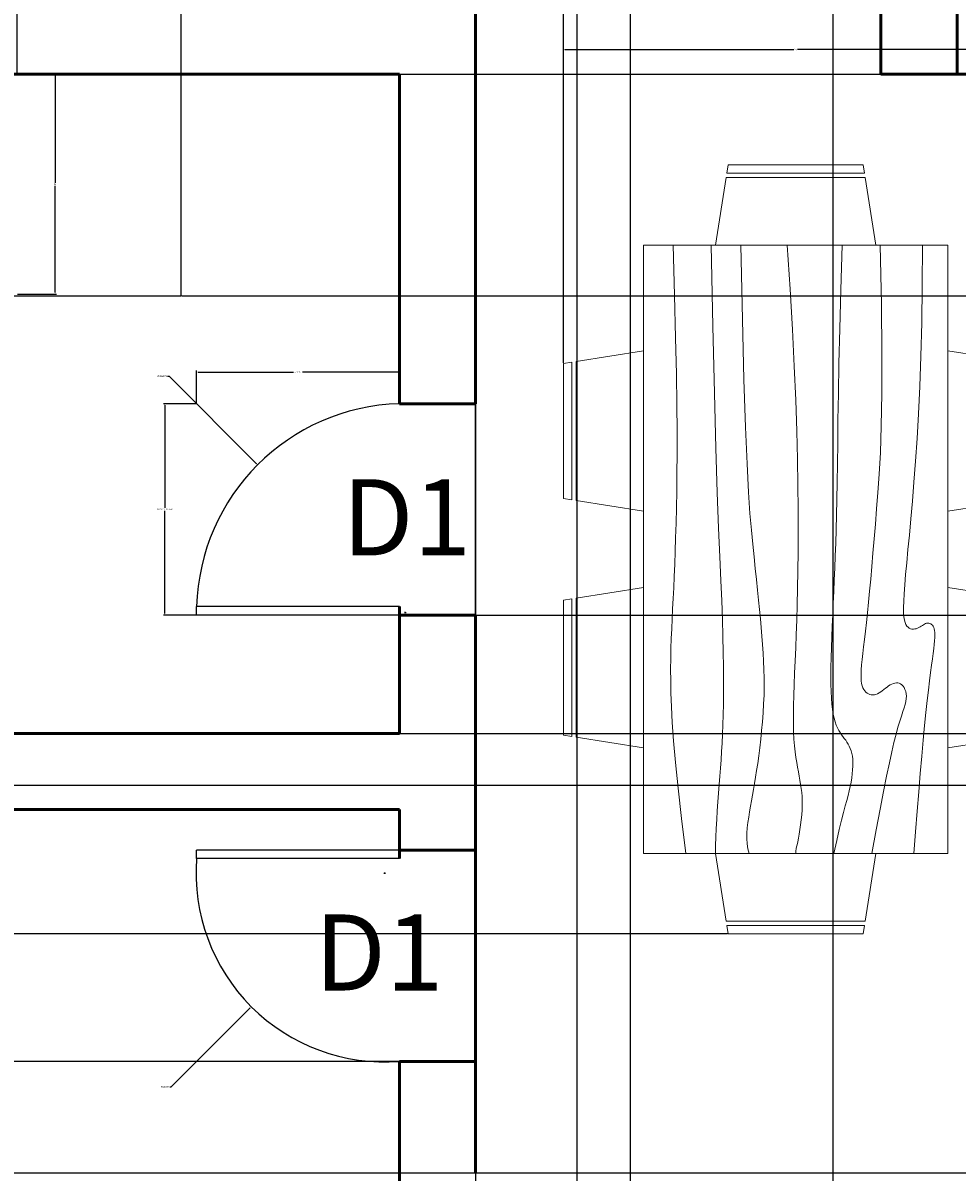
# Model space of a CAD drawing. Units: inches. Extents: x -3 to 419, y -430 to 101.
# Tile 3 of 5: x 118 to 229, y -259 to -123. Entities that reach past the tile are written whole.
import ezdxf

# ---------------------------------------------------------------- set-up
doc = ezdxf.new("R2010")
doc.units = ezdxf.units.IN
doc.header["$MEASUREMENT"] = 0
for name, color, linetype, lineweight in [('A-ANNO-DIMS', 2, 'Continuous', 18), ('A-ANNO-TEXT', 7, 'Continuous', 18), ('A-DOOR', 3, 'Continuous', 25), ('A-FLOR-CASE', 9, 'Continuous', 25), ('A-FURN', 8, 'Continuous', 18), ('A-WALL', 7, 'Continuous', 50)]:
    doc.layers.add(name, color=color, linetype=linetype, lineweight=lineweight)
doc.styles.get("Standard").update_dxf_attribs({"font": 'arial.ttf'})
doc.dimstyles.get("Standard").update_dxf_attribs({"dimtxt": 0.18, "dimasz": 0.18, "dimexe": 0.18, "dimexo": 0.0625, "dimgap": 0.09, "dimtad": 0, "dimtih": 1, "dimtoh": 1, "dimdec": 4, "dimzin": 0, "dimdsep": 46, "dimtxsty": 'Standard', "dimcen": 0.09, "dimadec": 0, "dimazin": 0, "dimtfac": 1, "dimtdec": 4, "dimtofl": 0, "dimtmove": 0, "dimatfit": 3, "dimfxl": 1, "dimtolj": 1, "dimtzin": 0, "dimarcsym": 0})

# ---------------------------------------------------------------- blocks, each defined once
blk = doc.blocks.new('Dining Set - 36 x 72 in.')
for p, q in [((-22, 27.5), (-22.1562, 26.50042)), ((-22, 27.5), (-6, 27.5)), ((-5.8437, 26.49966), (-6, 27.5)), ((6, 27.5), (5.8438, 26.50042)), ((6, 27.5), (22, 27.5)), ((22.1563, 26.49966), (22, 27.5)), ((-22.2343, 26.00059), (-23.4847, 17.99762)), ((-22.2304, 26), (-5.7608, 26)), ((-5.8416, 26.5), (-22.1534, 26.5)), ((-4.5152, 17.99762), (-5.7655, 25.99926)), ((5.7657, 26.00059), (4.5153, 17.99762)), ((5.7696, 26), (22.2392, 26)), ((22.1584, 26.5), (5.8466, 26.5)), ((23.4848, 17.99762), (22.2345, 25.99926)), ((36, 18), (-36, 18)), ((-36, 18), (-36, -18)), ((36, -18), (36, 18)), ((-44.0006, 8.23428), (-35.9976, 9.48474)), ((-44, 8.23041), (-44, -8.23915)), ((44.0006, 8.23428), (35.9976, 9.48474)), ((44, 8.23041), (44, -8.23915)), ((-45.5, 8), (-44.5004, 8.15617)), ((-45.5, 8), (-45.5, -8)), ((-44.5, -8.15843), (-44.5, 8.15338)), ((44.5, -8.15843), (44.5, 8.15338)), ((45.5, 8), (44.5005, 8.15617)), ((45.5, 8), (45.5, -8)), ((-44.4997, -8.15631), (-45.5, -8)), ((44.4997, -8.15631), (45.5, -8)), ((-35.9976, -9.48476), (-43.9993, -8.2345)), ((35.9976, -9.48476), (43.9993, -8.2345)), ((-36, -18), (36, -18)), ((-22.2343, -26.0006), (-23.4847, -17.99762)), ((-4.5152, -17.99762), (-5.7655, -25.99928)), ((5.7657, -26.0006), (4.5153, -17.99762)), ((23.4848, -17.99762), (22.2345, -25.99928)), ((-22.2304, -26), (-5.7608, -26)), ((-22, -27.5), (-22.1562, -26.50044)), ((-5.8416, -26.5), (-22.1534, -26.5)), ((-5.8437, -26.49967), (-6, -27.5)), ((5.7696, -26), (22.2392, -26)), ((6, -27.5), (5.8438, -26.50044)), ((22.1584, -26.5), (5.8466, -26.5)), ((22.1563, -26.49967), (22, -27.5)), ((-22, -27.5), (-6, -27.5)), ((6, -27.5), (22, -27.5))]:
    blk.add_line(p, q)
for points in [[(-36, 15), (-31.1772, 14.97754), (-26.8079, 14.91406), (-22.8538, 14.81543), (-19.276, 14.6875), (-16.0362, 14.53613), (-13.0957, 14.36718), (-10.4159, 14.18652), (-7.9583, 14), (-5.6904, 13.81315), (-3.6035, 13.63021), (-1.6954, 13.45508), (0.0365, 13.29166), (1.5945, 13.14388), (2.9811, 13.01562), (4.1988, 12.9108), (5.25, 12.83333), (6.1393, 12.78613), (6.8802, 12.76823), (7.4883, 12.77767), (7.9792, 12.8125), (8.3685, 12.87077), (8.6719, 12.95052), (8.9049, 13.0498), (9.0833, 13.16666), (9.2205, 13.29899), (9.3216, 13.44401), (9.3895, 13.59879), (9.4271, 13.76041), (9.4373, 13.92594), (9.4232, 14.09245), (9.3875, 14.257), (9.3333, 14.41666), (9.2638, 14.56917), (9.1836, 14.71484), (9.0975, 14.85465), (9.0104, 14.98958), (8.9272, 15.1206), (8.8529, 15.2487), (8.7922, 15.37483), (8.75, 15.5), (8.7305, 15.62467), (8.7344, 15.74739), (8.7617, 15.86621), (8.8125, 15.97916), (8.8867, 16.08431), (8.9844, 16.17968), (9.1055, 16.26334), (9.25, 16.33333), (9.4189, 16.38802), (9.6172, 16.42708), (9.8506, 16.45052), (10.125, 16.45833), (10.4463, 16.45052), (10.8203, 16.42708), (11.2529, 16.38802), (11.75, 16.33333), (12.3184, 16.26318), (12.9694, 16.17838), (13.7151, 16.07991), (14.5677, 15.96875), (15.5395, 15.84586), (16.6426, 15.71224), (17.8893, 15.56884), (19.2917, 15.41666), (20.859, 15.25667), (22.5879, 15.08984), (24.4721, 14.91715), (26.5052, 14.73958), (28.6809, 14.5581), (30.9929, 14.3737), (33.4347, 14.18733), (36, 14)], [(-36, 10), (-28.9766, 10.14274), (-23.1725, 10.20442), (-18.4241, 10.19775), (-14.5677, 10.13541), (-11.4399, 10.03011), (-8.877, 9.89453), (-6.7154, 9.74137), (-4.7917, 9.58333), (-2.9698, 9.43082), (-1.2246, 9.28515), (0.4415, 9.14534), (2.026, 9.01041), (3.5266, 8.87939), (4.9408, 8.7513), (6.266, 8.62516), (7.5, 8.5), (8.6411, 8.37549), (9.6914, 8.2539), (10.6538, 8.13818), (11.5312, 8.03125), (12.3267, 7.93603), (13.043, 7.85547), (13.6831, 7.79248), (14.25, 7.75), (14.7471, 7.7303), (15.1797, 7.73307), (15.5537, 7.75732), (15.875, 7.80208), (16.1494, 7.86637), (16.3828, 7.94922), (16.5811, 8.04964), (16.75, 8.16666), (16.8944, 8.29915), (17.0143, 8.44531), (17.1089, 8.60319), (17.1771, 8.77083), (17.218, 8.94629), (17.2305, 9.1276), (17.2137, 9.31282), (17.1667, 9.5), (17.0895, 9.6875), (16.987, 9.875), (16.8649, 10.0625), (16.7292, 10.25), (16.5856, 10.4375), (16.4401, 10.625), (16.2985, 10.8125), (16.1667, 11), (16.05, 11.18733), (15.9518, 11.3737), (15.8752, 11.5581), (15.8229, 11.73958), (15.798, 11.91715), (15.8034, 12.08984), (15.842, 12.25667), (15.9167, 12.41666), (16.0295, 12.56836), (16.1784, 12.70833), (16.3605, 12.83268), (16.5729, 12.9375), (16.8127, 13.01888), (17.0768, 13.07291), (17.3625, 13.0957), (17.6667, 13.08333), (17.9894, 13.03312), (18.3418, 12.94726), (18.7382, 12.82918), (19.1927, 12.68229), (19.7195, 12.51001), (20.3327, 12.31575), (21.0465, 12.10294), (21.875, 11.875), (22.8357, 11.63354), (23.959, 11.37304), (25.2786, 11.08618), (26.8282, 10.76562), (28.6414, 10.40405), (30.752, 9.99414), (33.1936, 9.52856), (36, 9)], [(-36, 5.5), (-30.7157, 5.3348), (-26.069, 5.20963), (-21.9946, 5.11767), (-18.4271, 5.05208), (-15.3009, 5.00602), (-12.5508, 4.97265), (-10.1112, 4.94515), (-7.9167, 4.91666), (-5.909, 4.88167), (-4.0586, 4.83984), (-2.3429, 4.79215), (-0.7396, 4.73958), (0.7739, 4.6831), (2.22, 4.6237), (3.6213, 4.56233), (5, 4.5), (6.373, 4.43782), (7.7344, 4.3776), (9.0723, 4.32129), (10.375, 4.27083), (11.6309, 4.22819), (12.8281, 4.19531), (13.9551, 4.17415), (15, 4.16666), (15.954, 4.17448), (16.819, 4.19791), (17.6001, 4.23698), (18.3021, 4.29166), (18.9299, 4.36198), (19.4883, 4.44791), (19.9823, 4.54948), (20.4167, 4.66666), (20.7969, 4.79899), (21.1302, 4.94401), (21.4245, 5.09879), (21.6875, 5.26041), (21.9271, 5.42594), (22.1511, 5.59245), (22.3672, 5.757), (22.5834, 5.91666), (22.8065, 6.06868), (23.0404, 6.21093), (23.2879, 6.34147), (23.5521, 6.45833), (23.8358, 6.55957), (24.142, 6.64323), (24.4735, 6.70735), (24.8334, 6.75), (25.2235, 6.76969), (25.642, 6.76692), (26.0858, 6.74267), (26.5521, 6.69791), (27.0379, 6.63362), (27.5404, 6.55078), (28.0565, 6.45036), (28.5834, 6.33333), (29.1242, 6.19987), (29.7071, 6.04687), (30.3661, 5.87044), (31.1354, 5.66666), (32.0493, 5.43164), (33.142, 5.16146), (34.4475, 4.85221), (36, 4.5)], [(-36, -1), (-30.7915, -0.6591), (-26.0195, -0.38216), (-21.6519, -0.16284), (-17.6563, 0.00521), (-14.0005, 0.12833), (-10.6523, 0.21289), (-7.5796, 0.26522), (-4.75, 0.29166), (-2.134, 0.29793), (0.2878, 0.28711), (2.5317, 0.26163), (4.6146, 0.22396), (6.5529, 0.17651), (8.3633, 0.12174), (10.0623, 0.06209), (11.6667, 0), (13.1899, -0.06201), (14.6341, -0.1211), (15.9982, -0.17432), (17.2813, -0.21875), (18.4823, -0.25147), (19.6003, -0.26953), (20.6343, -0.27002), (21.5834, -0.25), (22.4481, -0.20768), (23.2357, -0.14584), (23.9549, -0.06836), (24.6146, 0.02083), (25.2235, 0.11784), (25.7904, 0.21875), (26.3241, 0.31966), (26.8334, 0.41666), (27.3265, 0.50618), (27.8099, 0.58593), (28.2894, 0.65397), (28.7709, 0.70833), (29.2601, 0.74707), (29.763, 0.76823), (30.2855, 0.76985), (30.8334, 0.75), (31.4088, 0.70784), (31.9994, 0.64713), (32.589, 0.57275), (33.1615, 0.48958), (33.7008, 0.4025), (34.1908, 0.3164), (34.6153, 0.23616), (34.9584, 0.16666), (35.2099, 0.11165), (35.3848, 0.07031), (35.504, 0.04069), (35.5886, 0.02083), (35.6594, 0.00879), (35.7377, 0.0026), (35.8442, 0.00032), (36, 0)], [(-36, -6.5), (-27.1843, -6.31267), (-20.084, -6.1263), (-14.469, -5.9419), (-10.1094, -5.76042), (-6.7752, -5.58285), (-4.2363, -5.41016), (-2.2629, -5.24333), (-0.625, -5.08334), (0.8708, -4.93099), (2.2715, -4.78646), (3.5872, -4.64974), (4.8281, -4.52084), (6.0046, -4.39974), (7.127, -4.28646), (8.2053, -4.18099), (9.25, -4.08334), (10.2705, -3.99382), (11.2734, -3.91407), (12.2647, -3.84603), (13.25, -3.79167), (14.2354, -3.75293), (15.2266, -3.73177), (16.2295, -3.73015), (17.25, -3.75), (18.2912, -3.79248), (19.3451, -3.85547), (20.4009, -3.93604), (21.4479, -4.03125), (22.4754, -4.13819), (23.4727, -4.25391), (24.4289, -4.37549), (25.3334, -4.5), (26.1785, -4.62492), (26.9694, -4.74935), (27.7145, -4.87281), (28.4219, -4.99479), (29.1, -5.11483), (29.7572, -5.23242), (30.4016, -5.34709), (31.0417, -5.45834), (31.6837, -5.56437), (32.3262, -5.65821), (32.9658, -5.73153), (33.599, -5.77604), (34.2224, -5.78345), (34.8327, -5.74545), (35.4264, -5.65373), (36, -5.5)], [(-36, -10), (-26.4022, -9.81299), (-18.4675, -9.62891), (-11.9839, -9.45069), (-6.7396, -9.28125), (-2.5226, -9.12354), (0.8789, -8.98047), (3.6769, -8.85498), (6.0833, -8.75), (8.2767, -8.66765), (10.3021, -8.60677), (12.1712, -8.56543), (13.8958, -8.54167), (15.4876, -8.53353), (16.9583, -8.53907), (18.3197, -8.55632), (19.5834, -8.58334), (20.7616, -8.61841), (21.8685, -8.66081), (22.9188, -8.71004), (23.9271, -8.76563), (24.9081, -8.82707), (25.8763, -8.89388), (26.8465, -8.96558), (27.8334, -9.04167), (28.8474, -9.12118), (29.8828, -9.20117), (30.93, -9.27824), (31.9792, -9.34896), (33.0205, -9.40991), (34.0443, -9.45768), (35.0407, -9.48885), (36, -9.5)], [(-36, -14.5), (-30.0881, -14.33513), (-25.0332, -14.21224), (-20.7312, -14.12647), (-17.0781, -14.07292), (-13.97, -14.04671), (-11.3027, -14.04297), (-8.9724, -14.05681), (-6.875, -14.08334), (-4.9224, -14.11833), (-3.0905, -14.16016), (-1.3709, -14.20785), (0.2448, -14.26042), (1.7647, -14.3169), (3.1973, -14.3763), (4.5507, -14.43767), (5.8333, -14.5), (7.0554, -14.5621), (8.235, -14.62175), (9.3922, -14.67652), (10.5469, -14.72396), (11.7192, -14.76164), (12.929, -14.78711), (14.1965, -14.79794), (15.5417, -14.79167), (16.9933, -14.76424), (18.6152, -14.70508), (20.4804, -14.60197), (22.6615, -14.44271), (25.2312, -14.21509), (28.2624, -13.9069), (31.8277, -13.50594), (36, -13)]]:
    blk.add_lwpolyline(points)
blk = doc.blocks.new('DOOR-SWING-24IN')
for p, q in [((24, 1), (0, 1)), ((0, 0), (0, 1)), ((24, 0), (0, 0)), ((24, 1), (24, 0))]:
    blk.add_line(p, q)
blk.add_arc((24.7, 0.3), 24.71, 91.6273, 178.3727)
blk = doc.blocks.new('*D13')
at = {"layer": 'A-ANNO-DIMS', "color": 0, "lineweight": -2, "transparency": 16777216}
for p, q in [((138.49, -167.67), (134.62, -167.67)), ((134.8, -167.85), (134.8, -179.99)), ((134.8, -192.49), (134.8, -180.35)), ((138.49, -192.67), (134.62, -192.67))]:
    blk.add_line(p, q, dxfattribs=at)
at = {"layer": 'A-ANNO-DIMS', "color": 0, "transparency": 16777216}
for points in [[(134.77, -167.85), (134.83, -167.85), (134.8, -167.67)], [(134.77, -192.49), (134.83, -192.49), (134.8, -192.67)]]:
    blk.add_solid(points, dxfattribs=at)
at = {"layer": 'Defpoints', "color": 0, "transparency": 16777216}
for p in [(134.8, -167.67), (138.55, -167.67), (138.55, -192.67)]:
    blk.add_point(p, dxfattribs=at)
at = {"layer": 'A-ANNO-DIMS', "color": 0, "transparency": 16777216, "insert": (134.8, -180.17), "char_height": 0.18, "attachment_point": 5}
blk.add_mtext('\\A1;DOOR D1 25 TYP.', dxfattribs=at)
blk = doc.blocks.new('*D14')
at = {"layer": 'A-ANNO-DIMS', "color": 0, "lineweight": -2, "transparency": 16777216}
for p, q in [((138.55, -167.61), (138.55, -163.74)), ((138.73, -163.92), (150.02, -163.92)), ((162.37, -163.92), (151.08, -163.92)), ((162.55, -167.61), (162.55, -163.74))]:
    blk.add_line(p, q, dxfattribs=at)
at = {"layer": 'A-ANNO-DIMS', "color": 0, "transparency": 16777216}
for points in [[(138.73, -163.89), (138.73, -163.95), (138.55, -163.92)], [(162.37, -163.89), (162.37, -163.95), (162.55, -163.92)]]:
    blk.add_solid(points, dxfattribs=at)
at = {"layer": 'Defpoints', "color": 0, "transparency": 16777216}
for p in [(162.55, -163.92), (138.55, -167.67), (162.55, -167.67)]:
    blk.add_point(p, dxfattribs=at)
at = {"layer": 'A-ANNO-DIMS', "color": 0, "transparency": 16777216, "insert": (150.55, -163.92), "char_height": 0.18, "attachment_point": 5}
blk.add_mtext('\\A1;24 TYP.', dxfattribs=at)
blk = doc.blocks.new('*D18')
at = {"layer": 'A-ANNO-DIMS', "color": 0, "lineweight": -2, "transparency": 16777216}
for p, q in [((117.36, -128.7), (121.98, -128.7)), ((121.8, -128.88), (121.8, -141.52)), ((121.8, -154.52), (121.8, -141.88)), ((117.36, -154.7), (121.98, -154.7))]:
    blk.add_line(p, q, dxfattribs=at)
at = {"layer": 'A-ANNO-DIMS', "color": 0, "transparency": 16777216}
for points in [[(121.77, -128.88), (121.83, -128.88), (121.8, -128.7)], [(121.77, -154.52), (121.83, -154.52), (121.8, -154.7)]]:
    blk.add_solid(points, dxfattribs=at)
at = {"layer": 'Defpoints', "color": 0, "transparency": 16777216}
for p in [(117.3, -128.7), (121.8, -128.7), (117.3, -154.7)]:
    blk.add_point(p, dxfattribs=at)
at = {"layer": 'A-ANNO-DIMS', "color": 0, "transparency": 16777216, "insert": (121.8, -141.7), "char_height": 0.18, "attachment_point": 5}
blk.add_mtext('\\A1;26', dxfattribs=at)
blk = doc.blocks.new('*D20')
at = {"layer": 'A-ANNO-DIMS', "color": 0, "lineweight": -2, "transparency": 16777216}
for p, q in [((181.96, -139.34), (181.96, -125.57)), ((182.14, -125.75), (209.24, -125.75)), ((236.78, -125.75), (209.68, -125.75)), ((236.96, -139.34), (236.96, -125.57))]:
    blk.add_line(p, q, dxfattribs=at)
at = {"layer": 'A-ANNO-DIMS', "color": 0, "transparency": 16777216}
for points in [[(182.14, -125.72), (182.14, -125.78), (181.96, -125.75)], [(236.78, -125.72), (236.78, -125.78), (236.96, -125.75)]]:
    blk.add_solid(points, dxfattribs=at)
at = {"layer": 'Defpoints', "color": 0, "transparency": 16777216}
for p in [(236.96, -125.75), (181.96, -139.4), (236.96, -139.4)]:
    blk.add_point(p, dxfattribs=at)
at = {"layer": 'A-ANNO-DIMS', "color": 0, "transparency": 16777216, "insert": (209.46, -125.75), "char_height": 0.18, "attachment_point": 5}
blk.add_mtext('\\A1;55', dxfattribs=at)
blk = doc.blocks.new('*D26')
at = {"layer": 'A-ANNO-DIMS', "color": 0, "lineweight": -2, "transparency": 16777216}
for p, q in [((171.55, 12.25), (171.55, -429.67)), ((183.55, 12.25), (183.55, -429.67)), ((171.73, -429.49), (177.34, -429.49)), ((183.37, -429.49), (177.76, -429.49))]:
    blk.add_line(p, q, dxfattribs=at)
at = {"layer": 'A-ANNO-DIMS', "color": 0, "transparency": 16777216}
for points in [[(171.73, -429.46), (171.73, -429.52), (171.55, -429.49)], [(183.37, -429.46), (183.37, -429.52), (183.55, -429.49)]]:
    blk.add_solid(points, dxfattribs=at)
at = {"layer": 'Defpoints', "color": 0, "transparency": 16777216}
for p in [(171.55, 12.31), (183.55, 12.31), (183.55, -429.49)]:
    blk.add_point(p, dxfattribs=at)
at = {"layer": 'A-ANNO-DIMS', "color": 0, "transparency": 16777216, "insert": (177.55, -429.49), "char_height": 0.18, "attachment_point": 5}
blk.add_mtext('\\A1;12', dxfattribs=at)
blk = doc.blocks.new('*D37')
at = {"layer": 'A-ANNO-DIMS', "color": 0, "lineweight": -2, "transparency": 16777216}
for p, q in [((189.86, -65.75), (189.86, -429.67)), ((213.86, -65.75), (213.86, -429.67)), ((190.04, -429.49), (201.64, -429.49)), ((213.68, -429.49), (202.08, -429.49))]:
    blk.add_line(p, q, dxfattribs=at)
at = {"layer": 'A-ANNO-DIMS', "color": 0, "transparency": 16777216}
for points in [[(190.04, -429.46), (190.04, -429.52), (189.86, -429.49)], [(213.68, -429.46), (213.68, -429.52), (213.86, -429.49)]]:
    blk.add_solid(points, dxfattribs=at)
at = {"layer": 'Defpoints', "color": 0, "transparency": 16777216}
for p in [(189.86, -65.69), (213.86, -65.69), (213.86, -429.49)]:
    blk.add_point(p, dxfattribs=at)
at = {"layer": 'A-ANNO-DIMS', "color": 0, "transparency": 16777216, "insert": (201.86, -429.49), "char_height": 0.18, "attachment_point": 5}
blk.add_mtext('\\A1;24', dxfattribs=at)
blk = doc.blocks.new('*D39')
at = {"layer": 'A-ANNO-DIMS', "color": 0, "lineweight": -2, "transparency": 16777216}
for p, q in [((162.62, -192.67), (419.21, -192.67)), ((419.03, -192.85), (419.03, -199.5)), ((419.03, -206.51), (419.03, -199.86)), ((162.62, -206.69), (419.21, -206.69))]:
    blk.add_line(p, q, dxfattribs=at)
at = {"layer": 'A-ANNO-DIMS', "color": 0, "transparency": 16777216}
for points in [[(419, -192.85), (419.06, -192.85), (419.03, -192.67)], [(419, -206.51), (419.06, -206.51), (419.03, -206.69)]]:
    blk.add_solid(points, dxfattribs=at)
at = {"layer": 'Defpoints', "color": 0, "transparency": 16777216}
for p in [(162.55, -192.67), (162.55, -206.69), (419.03, -206.69)]:
    blk.add_point(p, dxfattribs=at)
at = {"layer": 'A-ANNO-DIMS', "color": 0, "transparency": 16777216, "insert": (419.03, -199.68), "char_height": 0.18, "attachment_point": 5}
blk.add_mtext('\\A1;14.014', dxfattribs=at)
blk = doc.blocks.new('*D40')
at = {"layer": 'A-ANNO-DIMS', "color": 0, "lineweight": -2, "transparency": 16777216}
for p, q in [((171.49, -245.49), (-3, -245.49)), ((-2.82, -245.67), (-2.82, -251.9)), ((-2.82, -258.51), (-2.82, -252.27)), ((171.49, -258.69), (-3, -258.69))]:
    blk.add_line(p, q, dxfattribs=at)
at = {"layer": 'A-ANNO-DIMS', "color": 0, "transparency": 16777216}
for points in [[(-2.85, -245.67), (-2.79, -245.67), (-2.82, -245.49)], [(-2.85, -258.51), (-2.79, -258.51), (-2.82, -258.69)]]:
    blk.add_solid(points, dxfattribs=at)
at = {"layer": 'Defpoints', "color": 0, "transparency": 16777216}
for p in [(171.55, -245.49), (-2.82, -258.69), (171.55, -258.69)]:
    blk.add_point(p, dxfattribs=at)
at = {"layer": 'A-ANNO-DIMS', "color": 0, "transparency": 16777216, "insert": (-2.82, -252.09), "char_height": 0.18, "attachment_point": 5}
blk.add_mtext('\\A1;13.2', dxfattribs=at)
blk = doc.blocks.new('*D48')
at = {"layer": 'A-ANNO-DIMS', "color": 0, "lineweight": -2, "transparency": 16777216}
for p, q in [((30.55, -128.62), (30.55, 101.37)), ((30.73, 101.19), (83.19, 101.19)), ((136.55, 101.19), (84.1, 101.19)), ((136.73, -128.62), (136.73, 101.37))]:
    blk.add_line(p, q, dxfattribs=at)
at = {"layer": 'A-ANNO-DIMS', "color": 0, "transparency": 16777216}
for points in [[(30.73, 101.22), (30.73, 101.16), (30.55, 101.19)], [(136.55, 101.22), (136.55, 101.16), (136.73, 101.19)]]:
    blk.add_solid(points, dxfattribs=at)
at = {"layer": 'Defpoints', "color": 0, "transparency": 16777216}
for p in [(136.73, 101.19), (30.55, -128.69), (136.73, -128.69)]:
    blk.add_point(p, dxfattribs=at)
at = {"layer": 'A-ANNO-DIMS', "color": 0, "transparency": 16777216, "insert": (83.64, 101.19), "char_height": 0.18, "attachment_point": 5}
blk.add_mtext('\\A1;106.18', dxfattribs=at)
blk = doc.blocks.new('*D50')
at = {"layer": 'A-ANNO-DIMS', "color": 0, "lineweight": -2, "transparency": 16777216}
for p, q in [((136.79, -128.69), (419.21, -128.69)), ((419.03, -128.87), (419.03, -141.62)), ((419.03, -154.74), (419.03, -141.99)), ((136.79, -154.92), (419.21, -154.92))]:
    blk.add_line(p, q, dxfattribs=at)
at = {"layer": 'A-ANNO-DIMS', "color": 0, "transparency": 16777216}
for points in [[(419, -128.87), (419.06, -128.87), (419.03, -128.69)], [(419, -154.74), (419.06, -154.74), (419.03, -154.92)]]:
    blk.add_solid(points, dxfattribs=at)
at = {"layer": 'Defpoints', "color": 0, "transparency": 16777216}
for p in [(136.73, -128.69), (136.73, -154.92), (419.03, -154.92)]:
    blk.add_point(p, dxfattribs=at)
at = {"layer": 'A-ANNO-DIMS', "color": 0, "transparency": 16777216, "insert": (419.03, -141.8), "char_height": 0.18, "attachment_point": 5}
blk.add_mtext('\\A1;26.24', dxfattribs=at)
blk = doc.blocks.new('*D52')
at = {"layer": 'A-ANNO-DIMS', "color": 0, "lineweight": -2, "transparency": 16777216}
for p, q in [((117.3, -128.64), (117.3, 101.37)), ((117.48, 101.19), (126.63, 101.19)), ((136.55, 101.19), (127.4, 101.19)), ((136.73, -128.62), (136.73, 101.37))]:
    blk.add_line(p, q, dxfattribs=at)
at = {"layer": 'A-ANNO-DIMS', "color": 0, "transparency": 16777216}
for points in [[(117.48, 101.22), (117.48, 101.16), (117.3, 101.19)], [(136.55, 101.22), (136.55, 101.16), (136.73, 101.19)]]:
    blk.add_solid(points, dxfattribs=at)
at = {"layer": 'Defpoints', "color": 0, "transparency": 16777216}
for p in [(136.73, 101.19), (117.3, -128.7), (136.73, -128.69)]:
    blk.add_point(p, dxfattribs=at)
at = {"layer": 'A-ANNO-DIMS', "color": 0, "transparency": 16777216, "insert": (127.01, 101.19), "char_height": 0.18, "attachment_point": 5}
blk.add_mtext('\\A1;19.43', dxfattribs=at)
blk = doc.blocks.new('*D53')
at = {"layer": 'A-ANNO-DIMS', "color": 0, "lineweight": -2, "transparency": 16777216}
for p, q in [((171.55, -167.61), (171.55, 101.37)), ((171.73, 101.19), (176.3, 101.19)), ((181.78, 101.19), (177.21, 101.19)), ((181.96, -162.84), (181.96, 101.37))]:
    blk.add_line(p, q, dxfattribs=at)
at = {"layer": 'A-ANNO-DIMS', "color": 0, "transparency": 16777216}
for points in [[(171.73, 101.22), (171.73, 101.16), (171.55, 101.19)], [(181.78, 101.22), (181.78, 101.16), (181.96, 101.19)]]:
    blk.add_solid(points, dxfattribs=at)
at = {"layer": 'Defpoints', "color": 0, "transparency": 16777216}
for p in [(181.96, 101.19), (181.96, -162.9), (171.55, -167.67)]:
    blk.add_point(p, dxfattribs=at)
at = {"layer": 'A-ANNO-DIMS', "color": 0, "transparency": 16777216, "insert": (176.76, 101.19), "char_height": 0.18, "attachment_point": 5}
blk.add_mtext('\\A1;10.407', dxfattribs=at)
blk = doc.blocks.new('*D54')
at = {"layer": 'A-ANNO-DIMS', "color": 0, "lineweight": -2, "transparency": 16777216}
for p, q in [((201.4, -230.4), (-3, -230.4)), ((-2.82, -230.58), (-2.82, -244.36)), ((-2.82, -258.51), (-2.82, -244.72)), ((199.03, -258.69), (-3, -258.69))]:
    blk.add_line(p, q, dxfattribs=at)
at = {"layer": 'A-ANNO-DIMS', "color": 0, "transparency": 16777216}
for points in [[(-2.85, -230.58), (-2.79, -230.58), (-2.82, -230.4)], [(-2.85, -258.51), (-2.79, -258.51), (-2.82, -258.69)]]:
    blk.add_solid(points, dxfattribs=at)
at = {"layer": 'Defpoints', "color": 0, "transparency": 16777216}
for p in [(201.46, -230.4), (-2.82, -258.69), (199.09, -258.69)]:
    blk.add_point(p, dxfattribs=at)
at = {"layer": 'A-ANNO-DIMS', "color": 0, "transparency": 16777216, "insert": (-2.82, -244.54), "char_height": 0.18, "attachment_point": 5}
blk.add_mtext('\\A1;28.286', dxfattribs=at)
blk = doc.blocks.new('*D55')
at = {"layer": 'A-ANNO-DIMS', "color": 0, "lineweight": -2, "transparency": 16777216}
for p, q in [((255.33, -212.85), (-3, -212.85)), ((-2.82, -213.03), (-2.82, -235.59)), ((-2.82, -258.51), (-2.82, -235.95)), ((269.16, -258.69), (-3, -258.69))]:
    blk.add_line(p, q, dxfattribs=at)
at = {"layer": 'A-ANNO-DIMS', "color": 0, "transparency": 16777216}
for points in [[(-2.85, -213.03), (-2.79, -213.03), (-2.82, -212.85)], [(-2.85, -258.51), (-2.79, -258.51), (-2.82, -258.69)]]:
    blk.add_solid(points, dxfattribs=at)
at = {"layer": 'Defpoints', "color": 0, "transparency": 16777216}
for p in [(255.4, -212.85), (-2.82, -258.69), (269.22, -258.69)]:
    blk.add_point(p, dxfattribs=at)
at = {"layer": 'A-ANNO-DIMS', "color": 0, "transparency": 16777216, "insert": (-2.82, -235.77), "char_height": 0.18, "attachment_point": 5}
blk.add_mtext('\\A1;45.83', dxfattribs=at)
blk = doc.blocks.new('*D60')
at = {"layer": 'A-ANNO-DIMS', "color": 0, "lineweight": -2, "transparency": 16777216}
for p, q in [((162.55, -245.55), (162.55, -429.67)), ((118.01, -284.25), (118.01, -429.67)), ((118.19, -429.49), (139.88, -429.49)), ((162.37, -429.49), (140.68, -429.49))]:
    blk.add_line(p, q, dxfattribs=at)
at = {"layer": 'A-ANNO-DIMS', "color": 0, "transparency": 16777216}
for points in [[(118.19, -429.46), (118.19, -429.52), (118.01, -429.49)], [(162.37, -429.46), (162.37, -429.52), (162.55, -429.49)]]:
    blk.add_solid(points, dxfattribs=at)
at = {"layer": 'Defpoints', "color": 0, "transparency": 16777216}
for p in [(162.55, -245.49), (118.01, -284.19), (162.55, -429.49)]:
    blk.add_point(p, dxfattribs=at)
at = {"layer": 'A-ANNO-DIMS', "color": 0, "transparency": 16777216, "insert": (140.28, -429.49), "char_height": 0.18, "attachment_point": 5}
blk.add_mtext('\\A1;44.55', dxfattribs=at)
blk = doc.blocks.new('*D67')
at = {"layer": 'A-ANNO-DIMS', "color": 0, "lineweight": -2, "transparency": 16777216}
for p, q in [((162.46, -255.14), (162.64, -255.14)), ((162.55, -255.23), (162.55, -255.05)), ((206.26, -298.85), (190, -282.59)), ((206.44, -298.85), (206.26, -298.85))]:
    blk.add_line(p, q, dxfattribs=at)
at = {"layer": 'A-ANNO-DIMS', "color": 0, "transparency": 16777216}
blk.add_solid([(190.02, -282.57), (189.97, -282.61), (189.87, -282.46)], dxfattribs=at)
at = {"layer": 'Defpoints', "color": 0, "transparency": 16777216}
for p in [(162.55, -255.14), (189.87, -282.46)]:
    blk.add_point(p, dxfattribs=at)
at = {"layer": 'A-ANNO-DIMS', "color": 0, "transparency": 16777216, "insert": (206.99, -298.85), "char_height": 0.18, "attachment_point": 5}
blk.add_mtext('\\A1;R38.636', dxfattribs=at)
blk = doc.blocks.new('*D70')
at = {"layer": 'A-ANNO-DIMS', "color": 0, "lineweight": -2, "transparency": 16777216}
for p, q in [((135.12, -164.41), (135.3, -164.41)), ((135.3, -164.41), (145.65, -174.77)), ((163.16, -192.37), (163.34, -192.37)), ((163.25, -192.46), (163.25, -192.28))]:
    blk.add_line(p, q, dxfattribs=at)
at = {"layer": 'A-ANNO-DIMS', "color": 0, "transparency": 16777216}
blk.add_solid([(145.68, -174.75), (145.63, -174.79), (145.78, -174.9)], dxfattribs=at)
at = {"layer": 'Defpoints', "color": 0, "transparency": 16777216}
for p in [(145.78, -174.9), (163.25, -192.37)]:
    blk.add_point(p, dxfattribs=at)
at = {"layer": 'A-ANNO-DIMS', "color": 0, "transparency": 16777216, "insert": (134.46, -164.41), "char_height": 0.18, "attachment_point": 5}
blk.add_mtext('\\A1;2X R24.71', dxfattribs=at)
blk = doc.blocks.new('*D72')
at = {"layer": 'A-ANNO-DIMS', "color": 0, "lineweight": -2, "transparency": 16777216}
for p, q in [((160.82, -223.31), (160.82, -223.13)), ((160.73, -223.22), (160.91, -223.22)), ((135.55, -248.49), (144.9, -239.14)), ((135.37, -248.49), (135.55, -248.49))]:
    blk.add_line(p, q, dxfattribs=at)
at = {"layer": 'A-ANNO-DIMS', "color": 0, "transparency": 16777216}
blk.add_solid([(144.88, -239.12), (144.92, -239.16), (145.03, -239.01)], dxfattribs=at)
at = {"layer": 'Defpoints', "color": 0, "transparency": 16777216}
for p in [(160.82, -223.22), (145.03, -239.01)]:
    blk.add_point(p, dxfattribs=at)
at = {"layer": 'A-ANNO-DIMS', "color": 0, "transparency": 16777216, "insert": (134.82, -248.49), "char_height": 0.18, "attachment_point": 5}
blk.add_mtext('\\A1;R22.337', dxfattribs=at)

msp = doc.modelspace()

# ---------------------------------------------------------------- linework, layer by layer
at = {"layer": 'A-DOOR'}
for p, q in [((171.5532, -192.6713), (171.5532, -167.6713)), ((162.5532, -220.4865), (138.5532, -220.4865)), ((138.5532, -221.4865), (138.5532, -220.4865)), ((162.5532, -221.4865), (138.5532, -221.4865)), ((162.5532, -220.4865), (162.5532, -221.4865))]:
    msp.add_line(p, q, dxfattribs=at)
msp.add_arc((160.8227, -223.217), 22.3366, 175.556582, 274.443418, dxfattribs=at)
at = {"layer": 'A-FLOR-CASE'}
for p, q in [((136.73, -154.9237), (136.73, -128.6853)), ((55.004, -154.9237), (136.73, -154.9237))]:
    msp.add_line(p, q, dxfattribs=at)
at = {"layer": 'A-WALL'}
for p, q in [((171.5532, -167.6713), (171.5532, -111.2695)), ((228.5532, -128.6853), (228.5532, -117.277)), ((219.5532, -119.6853), (219.5532, -128.6853)), ((30.5532, -128.6853), (162.5532, -128.6853)), ((162.5532, -128.6853), (162.5532, -167.6713)), ((219.5532, -128.6853), (228.5532, -128.6853)), ((228.5532, -128.6853), (336.5532, -128.6853)), ((162.5532, -167.6713), (171.5532, -167.6713)), ((162.5532, -206.6853), (162.5532, -191.6713)), ((162.5532, -192.6713), (171.5532, -192.6713)), ((171.5532, -258.6853), (171.5532, -192.6713)), ((30.5532, -206.6853), (162.5532, -206.6853)), ((30.5532, -215.6853), (162.5532, -215.6853)), ((162.5532, -221.4865), (162.5532, -215.6853)), ((162.5532, -220.4865), (171.5532, -220.4865)), ((162.5532, -267.6853), (162.5532, -245.4865)), ((162.5532, -245.4865), (171.5532, -245.4865))]:
    msp.add_line(p, q, dxfattribs=at)

# ---------------------------------------------------------------- block references
at = {"layer": 'A-DOOR'}
msp.add_blockref('DOOR-SWING-24IN', (138.553, -192.6718), dxfattribs=at)
at = {"layer": 'A-FURN', "rotation": 270}
msp.add_blockref('Dining Set - 36 x 72 in.', (209.4598, -184.8988), dxfattribs=at)

# ---------------------------------------------------------------- texts
at = {"layer": 'A-ANNO-TEXT', "char_height": 9, "attachment_point": 1}
for width, insert in [(15.43411, (155.7744, -176.6084)), (16.342001, (152.5109, -228.0959))]:
    msp.add_mtext_dynamic_manual_height_columns('D1', width=width, gutter_width=45, heights=[0], dxfattribs=dict(at, insert=insert))

# ---------------------------------------------------------------- dimensions: what is measured, and where the dimension line sits
at = {"layer": 'A-ANNO-DIMS'}
for base, p1, p2, override, picture, middle in [((136.73, 101.1903), (30.5532, -128.6853), (136.73, -128.6853), {"dimdec": 2, "dimlfac": 1, "dimrnd": 0, "dimzin": 0, "dimdsep": 46, "dimlunit": 2}, '*D48', (83.6416, 101.1903)), ((136.73, 101.1903), (117.2993, -128.7009), (136.73, -128.6853), {"dimdec": 2, "dimlfac": 1, "dimrnd": 0, "dimzin": 0, "dimdsep": 46, "dimlunit": 2}, '*D52', (127.0147, 101.1903)), ((181.9598, 101.1903), (171.5532, -167.6713), (181.9598, -162.8988), {"dimdec": 3, "dimlfac": 1, "dimrnd": 0, "dimzin": 0, "dimdsep": 46, "dimlunit": 2}, '*D53', (176.7565, 101.1903)), ((183.5532, -429.4854), (171.5532, 12.3147), (183.5532, 12.3147), {"dimdec": 0, "dimlfac": 1, "dimrnd": 0, "dimzin": 0, "dimdsep": 46, "dimlunit": 2}, '*D26', (177.5532, -429.4854)), ((213.8603, -429.4854), (189.8603, -65.6853), (213.8603, -65.6853), {"dimdec": 0, "dimlfac": 1, "dimrnd": 0, "dimzin": 0, "dimdsep": 46, "dimlunit": 2}, '*D37', (201.8603, -429.4854)), ((236.9598, -125.7488), (181.9598, -139.3988), (236.9598, -139.3988), {"dimdec": 0, "dimlfac": 1, "dimrnd": 0, "dimzin": 0, "dimdsep": 46, "dimlunit": 2}, '*D20', (209.4598, -125.7488)), ((162.5532, -429.4854), (118.0057, -284.1853), (162.5532, -245.4865), {"dimdec": 2, "dimlfac": 1, "dimrnd": 0, "dimzin": 0, "dimdsep": 46, "dimlunit": 2}, '*D60', (140.2794, -429.4854))]:
    dim = msp.add_linear_dim(base=base, p1=p1, p2=p2, dimstyle='Standard', override=override, dxfattribs=at)
    dim.commit()
    dim.dimension.update_dxf_attribs({"geometry": picture, "text_midpoint": middle})
for base, p1, p2, override, picture, middle in [((121.7993, -128.7009), (117.2993, -154.7009), (117.2993, -128.7009), {"dimdec": 0, "dimlfac": 1, "dimrnd": 0, "dimzin": 0, "dimdsep": 46, "dimlunit": 2}, '*D18', (121.7993, -141.7009)), ((419.0271, -154.9237), (136.73, -128.6853), (136.73, -154.9237), {"dimdec": 2, "dimlfac": 1, "dimrnd": 0, "dimzin": 0, "dimdsep": 46, "dimlunit": 2}, '*D50', (419.0271, -141.8045)), ((419.0271, -206.6853), (162.5532, -192.6713), (162.5532, -206.6853), {"dimdec": 3, "dimlfac": 1, "dimrnd": 0, "dimzin": 0, "dimdsep": 46, "dimlunit": 2}, '*D39', (419.0271, -199.6783)), ((-2.8238, -258.6853), (255.3974, -212.8529), (269.2198, -258.6853), {"dimdec": 2, "dimlfac": 1, "dimrnd": 0, "dimzin": 0, "dimdsep": 46, "dimlunit": 2}, '*D55', (-2.8238, -235.7691)), ((-2.82381, -258.68531), (201.45976, -230.39884), (199.09163, -258.68531), {"dimdec": 3, "dimlfac": 1, "dimrnd": 0, "dimzin": 0, "dimdsep": 46, "dimlunit": 2}, '*D54', (-2.82381, -244.54208)), ((-2.8238, -258.6853), (171.5532, -245.4865), (171.5532, -258.6853), {"dimdec": 1, "dimlfac": 1, "dimrnd": 0, "dimzin": 0, "dimdsep": 46, "dimlunit": 2}, '*D40', (-2.8238, -252.0859))]:
    dim = msp.add_linear_dim(base=base, p1=p1, p2=p2, angle=90, dimstyle='Standard', override=override, dxfattribs=at)
    dim.commit()
    dim.dimension.update_dxf_attribs({"geometry": picture, "text_midpoint": middle})
dim = msp.add_radius_dim(center=(163.255, -192.373), mpoint=(145.7812, -174.8992), text='2X <>', dimstyle='Standard', override={"dimdec": 2, "dimlfac": 1, "dimrnd": 0, "dimzin": 0, "dimdsep": 46, "dimlunit": 2}, dxfattribs=at)
dim.commit()
dim.dimension.update_dxf_attribs({"geometry": '*D70', "text_midpoint": (134.4595, -164.4148), "dimtype": 164})
dim = msp.add_linear_dim(base=(162.5532, -163.9213), p1=(138.5532, -167.6713), p2=(162.5532, -167.6713), text='<> TYP.', dimstyle='Standard', override={"dimdec": 0, "dimlfac": 1, "dimrnd": 0, "dimzin": 0, "dimdsep": 46, "dimlunit": 2}, dxfattribs=at)
dim.commit()
dim.dimension.update_dxf_attribs({"geometry": '*D14', "text_midpoint": (150.5532, -163.9213)})
dim = msp.add_linear_dim(base=(134.8032, -167.6713), p1=(138.5532, -192.6713), p2=(138.5532, -167.6713), angle=90, text='DOOR D1 <> TYP.', dimstyle='Standard', override={"dimdec": 0, "dimlfac": 1, "dimrnd": 0, "dimzin": 0, "dimdsep": 46, "dimlunit": 2}, dxfattribs=at)
dim.commit()
dim.dimension.update_dxf_attribs({"geometry": '*D13', "text_midpoint": (134.8032, -180.1713)})
for center, mpoint, picture, middle in [((160.8227, -223.217), (145.028, -239.011), '*D72', (134.8214, -248.4875)), ((162.5485, -255.1422), (189.868, -282.462), '*D67', (206.9894, -298.8539))]:
    dim = msp.add_radius_dim(center=center, mpoint=mpoint, dimstyle='Standard', override={"dimdec": 3, "dimlfac": 1, "dimrnd": 0, "dimzin": 0, "dimdsep": 46, "dimlunit": 2}, dxfattribs=at)
    dim.commit()
    dim.dimension.update_dxf_attribs({"geometry": picture, "text_midpoint": middle, "dimtype": 164})

doc.saveas('drawing.dxf')
